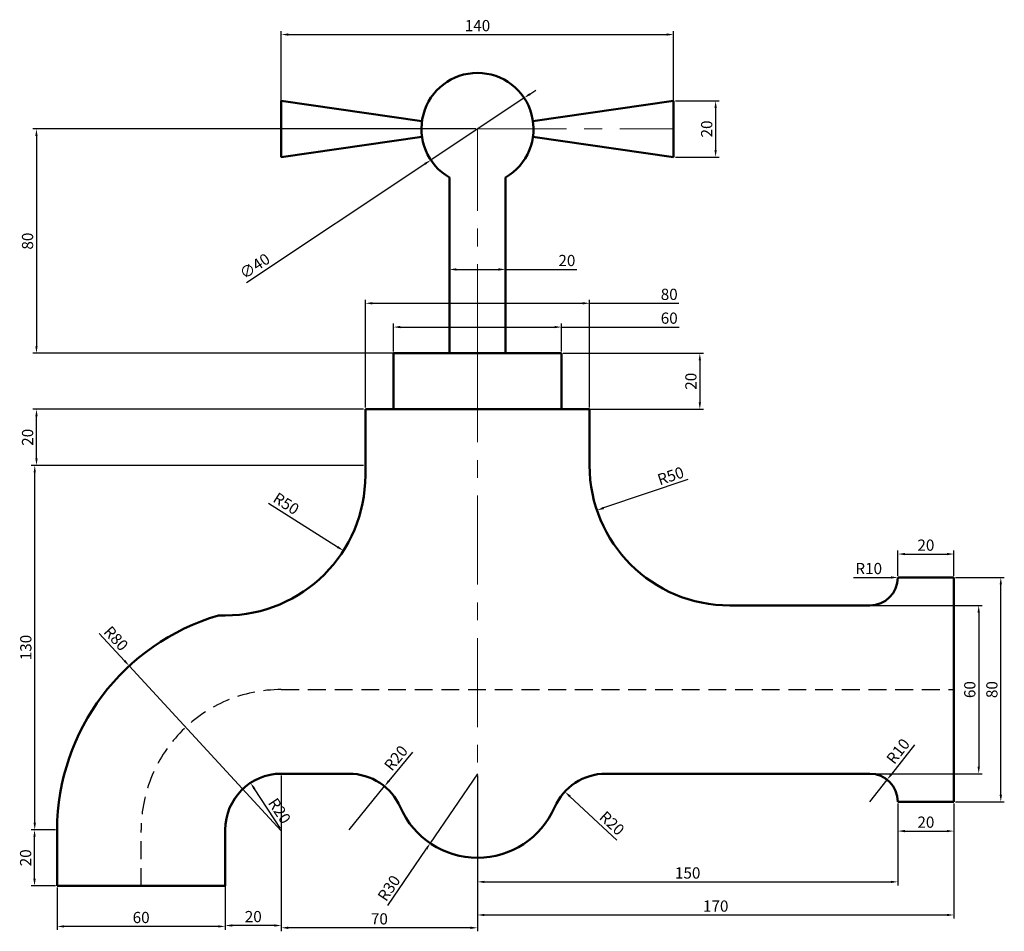
# Model space of a CAD drawing. Units: millimetres. Extents: x 1591 to 1942, y 1200 to 1525.
import ezdxf

# ---------------------------------------------------------------- set-up
doc = ezdxf.new("R2010")
doc.units = ezdxf.units.MM
doc.linetypes.add('CENTER', pattern=[50.8, 31.75, -6.35, 6.35, -6.35])
doc.linetypes.add('HIDDEN', pattern=[9.525, 6.35, -3.175])
for name, color, linetype, lineweight in [('M-CNTR', 1, 'CENTER', 18), ('M-DIMS', 2, 'Continuous', 25), ('M-HIDN', 4, 'HIDDEN', 25), ('M-OUTL', 7, 'Continuous', 50)]:
    doc.layers.add(name, color=color, linetype=linetype, lineweight=lineweight)
doc.styles.get("Standard").update_dxf_attribs({"font": 'arial.ttf'})
doc.dimstyles.new('ISO-25', dxfattribs={"dimtxt": 4, "dimasz": 2.5, "dimexe": 1.25, "dimexo": 0.625, "dimtad": 1, "dimtxsty": 'Standard', "dimcen": 2.5, "dimadec": 0, "dimazin": 0, "dimtfac": 1, "dimtmove": 0, "dimatfit": 3, "dimfxl": 1, "dimarcsym": 0})

# ---------------------------------------------------------------- blocks, each defined once
blk = doc.blocks.new('*D1')
at = {"layer": 'Defpoints', "color": 0, "transparency": 16777216}
for p in [(1923.89, 1325.86), (1940.62, 1325.86), (1923.89, 1245.86)]:
    blk.add_point(p, dxfattribs=at)
at = {"layer": 'M-DIMS', "color": 0, "lineweight": -2, "transparency": 16777216}
for p, q in [((1924.51, 1325.86), (1941.87, 1325.86)), ((1940.62, 1248.36), (1940.62, 1323.36)), ((1924.51, 1245.86), (1941.87, 1245.86))]:
    blk.add_line(p, q, dxfattribs=at)
at = {"layer": 'M-DIMS', "color": 0, "transparency": 16777216}
for points in [[(1940.21, 1323.36), (1941.04, 1323.36), (1940.62, 1325.86)], [(1940.21, 1248.36), (1941.04, 1248.36), (1940.62, 1245.86)]]:
    blk.add_solid(points, dxfattribs=at)
at = {"layer": 'M-DIMS', "color": 0, "transparency": 16777216, "insert": (1937.96, 1285.86), "char_height": 4, "attachment_point": 5, "rotation": 90}
blk.add_mtext('80', dxfattribs=at)
blk = doc.blocks.new('*D2')
at = {"layer": 'Defpoints', "color": 0, "transparency": 16777216}
for p in [(1663.89, 1362.31), (1706.04, 1335.42)]:
    blk.add_point(p, dxfattribs=at)
at = {"layer": 'M-DIMS', "color": 0, "lineweight": -2, "transparency": 16777216}
blk.add_line((1679.37, 1352.43), (1703.94, 1336.76), dxfattribs=at)
at = {"layer": 'M-DIMS', "color": 0, "transparency": 16777216}
blk.add_solid([(1704.16, 1337.11), (1703.71, 1336.41), (1706.04, 1335.42)], dxfattribs=at)
at = {"layer": 'M-DIMS', "color": 0, "transparency": 16777216, "insert": (1685.35, 1351.78), "char_height": 4, "attachment_point": 5, "rotation": 327.4692}
blk.add_mtext('R50', dxfattribs=at)
blk = doc.blocks.new('*D3')
at = {"layer": 'Defpoints', "color": 0, "transparency": 16777216}
for p in [(1843.89, 1365.86), (1796.52, 1349.85)]:
    blk.add_point(p, dxfattribs=at)
at = {"layer": 'M-DIMS', "color": 0, "lineweight": -2, "transparency": 16777216}
blk.add_line((1828.96, 1360.81), (1798.89, 1350.65), dxfattribs=at)
at = {"layer": 'M-DIMS', "color": 0, "transparency": 16777216}
blk.add_solid([(1798.76, 1351.04), (1799.02, 1350.25), (1796.52, 1349.85)], dxfattribs=at)
at = {"layer": 'M-DIMS', "color": 0, "transparency": 16777216, "insert": (1822.99, 1361.61), "char_height": 4, "attachment_point": 5, "rotation": 18.6803}
blk.add_mtext('R50', dxfattribs=at)
blk = doc.blocks.new('*D4')
at = {"layer": 'Defpoints', "color": 0, "transparency": 16777216}
for p in [(1785.05, 1249.46), (1799.71, 1235.86)]:
    blk.add_point(p, dxfattribs=at)
at = {"layer": 'M-DIMS', "color": 0, "lineweight": -2, "transparency": 16777216}
blk.add_line((1803.67, 1232.19), (1786.89, 1247.76), dxfattribs=at)
at = {"layer": 'M-DIMS', "color": 0, "transparency": 16777216}
blk.add_solid([(1787.17, 1248.07), (1786.6, 1247.46), (1785.05, 1249.46)], dxfattribs=at)
at = {"layer": 'M-DIMS', "color": 0, "transparency": 16777216, "insert": (1801.53, 1237.82), "char_height": 4, "attachment_point": 5, "rotation": 317.1429}
blk.add_mtext('R20', dxfattribs=at)
blk = doc.blocks.new('*D5')
at = {"layer": 'Defpoints', "color": 0, "transparency": 16777216}
for p in [(1720.7, 1251.36), (1708.06, 1235.86)]:
    blk.add_point(p, dxfattribs=at)
at = {"layer": 'M-DIMS', "color": 0, "lineweight": -2, "transparency": 16777216}
for p, q in [((1730.68, 1263.6), (1722.28, 1253.3)), ((1708.06, 1235.86), (1720.7, 1251.36))]:
    blk.add_line(p, q, dxfattribs=at)
at = {"layer": 'M-DIMS', "color": 0, "transparency": 16777216}
blk.add_solid([(1721.96, 1253.56), (1722.6, 1253.04), (1720.7, 1251.36)], dxfattribs=at)
at = {"layer": 'M-DIMS', "color": 0, "transparency": 16777216, "insert": (1725.2, 1261.11), "char_height": 4, "attachment_point": 5, "rotation": 50.8113}
blk.add_mtext('R20', dxfattribs=at)
blk = doc.blocks.new('*D6')
at = {"layer": 'Defpoints', "color": 0, "transparency": 16777216}
for p in [(1893.89, 1325.86), (1903.89, 1325.86)]:
    blk.add_point(p, dxfattribs=at)
at = {"layer": 'M-DIMS', "color": 0, "lineweight": -2, "transparency": 16777216}
blk.add_line((1888.09, 1325.86), (1901.39, 1325.86), dxfattribs=at)
at = {"layer": 'M-DIMS', "color": 0, "transparency": 16777216}
blk.add_solid([(1901.39, 1326.28), (1901.39, 1325.44), (1903.89, 1325.86)], dxfattribs=at)
at = {"layer": 'M-DIMS', "color": 0, "transparency": 16777216, "insert": (1893.49, 1328.53), "char_height": 4, "attachment_point": 5}
blk.add_mtext('R10', dxfattribs=at)
blk = doc.blocks.new('*D7')
at = {"layer": 'Defpoints', "color": 0, "transparency": 16777216}
for p in [(1753.89, 1255.86), (1737.03, 1231.05)]:
    blk.add_point(p, dxfattribs=at)
at = {"layer": 'M-DIMS', "color": 0, "lineweight": -2, "transparency": 16777216}
for p, q in [((1753.89, 1255.86), (1737.03, 1231.05)), ((1721.9, 1208.79), (1735.62, 1228.98))]:
    blk.add_line(p, q, dxfattribs=at)
at = {"layer": 'M-DIMS', "color": 0, "transparency": 16777216}
blk.add_solid([(1735.28, 1229.21), (1735.97, 1228.75), (1737.03, 1231.05)], dxfattribs=at)
at = {"layer": 'M-DIMS', "color": 0, "transparency": 16777216, "insert": (1722.73, 1214.75), "char_height": 4, "attachment_point": 5, "rotation": 55.803}
blk.add_mtext('R30', dxfattribs=at)
blk = doc.blocks.new('*D8')
at = {"layer": 'Defpoints', "color": 0, "transparency": 16777216}
for p in [(1672.91, 1252.58), (1683.89, 1235.86)]:
    blk.add_point(p, dxfattribs=at)
at = {"layer": 'M-DIMS', "color": 0, "lineweight": -2, "transparency": 16777216}
blk.add_line((1683.58, 1236.34), (1674.28, 1250.49), dxfattribs=at)
at = {"layer": 'M-DIMS', "color": 0, "transparency": 16777216}
blk.add_solid([(1674.63, 1250.72), (1673.93, 1250.26), (1672.91, 1252.58)], dxfattribs=at)
at = {"layer": 'M-DIMS', "color": 0, "transparency": 16777216, "insert": (1682.84, 1242.31), "char_height": 4, "attachment_point": 5, "rotation": 303.2913}
blk.add_mtext('R20', dxfattribs=at)
blk = doc.blocks.new('*D9')
at = {"layer": 'Defpoints', "color": 0, "transparency": 16777216}
for p in [(1629.63, 1294.31), (1683.89, 1235.52)]:
    blk.add_point(p, dxfattribs=at)
at = {"layer": 'M-DIMS', "color": 0, "lineweight": -2, "transparency": 16777216}
for p, q in [((1618.92, 1305.92), (1627.93, 1296.15)), ((1683.89, 1235.52), (1629.63, 1294.31))]:
    blk.add_line(p, q, dxfattribs=at)
at = {"layer": 'M-DIMS', "color": 0, "transparency": 16777216}
blk.add_solid([(1628.24, 1296.43), (1627.63, 1295.87), (1629.63, 1294.31)], dxfattribs=at)
at = {"layer": 'M-DIMS', "color": 0, "transparency": 16777216, "insert": (1624.54, 1303.76), "char_height": 4, "attachment_point": 5, "rotation": 312.7056}
blk.add_mtext('R80', dxfattribs=at)
blk = doc.blocks.new('*D10')
at = {"layer": 'Defpoints', "color": 0, "transparency": 16777216}
for p in [(1603.89, 1215.86), (1663.89, 1215.86), (1603.89, 1201.38)]:
    blk.add_point(p, dxfattribs=at)
at = {"layer": 'M-DIMS', "color": 0, "lineweight": -2, "transparency": 16777216}
for p, q in [((1603.89, 1215.24), (1603.89, 1200.13)), ((1663.89, 1215.24), (1663.89, 1200.13)), ((1661.39, 1201.38), (1606.39, 1201.38))]:
    blk.add_line(p, q, dxfattribs=at)
at = {"layer": 'M-DIMS', "color": 0, "transparency": 16777216}
for points in [[(1606.39, 1201.8), (1606.39, 1200.97), (1603.89, 1201.38)], [(1661.39, 1201.8), (1661.39, 1200.97), (1663.89, 1201.38)]]:
    blk.add_solid(points, dxfattribs=at)
at = {"layer": 'M-DIMS', "color": 0, "transparency": 16777216, "insert": (1633.89, 1204.05), "char_height": 4, "attachment_point": 5}
blk.add_mtext('60', dxfattribs=at)
blk = doc.blocks.new('*D11')
at = {"layer": 'Defpoints', "color": 0, "transparency": 16777216}
for p in [(1683.89, 1255.86), (1663.89, 1235.86), (1663.89, 1201.7)]:
    blk.add_point(p, dxfattribs=at)
at = {"layer": 'M-DIMS', "color": 0, "lineweight": -2, "transparency": 16777216}
for p, q in [((1683.89, 1255.24), (1683.89, 1200.45)), ((1663.89, 1235.24), (1663.89, 1200.45)), ((1681.39, 1201.7), (1666.39, 1201.7))]:
    blk.add_line(p, q, dxfattribs=at)
at = {"layer": 'M-DIMS', "color": 0, "transparency": 16777216}
for points in [[(1666.39, 1202.12), (1666.39, 1201.29), (1663.89, 1201.7)], [(1681.39, 1202.12), (1681.39, 1201.29), (1683.89, 1201.7)]]:
    blk.add_solid(points, dxfattribs=at)
at = {"layer": 'M-DIMS', "color": 0, "transparency": 16777216, "insert": (1673.89, 1204.37), "char_height": 4, "attachment_point": 5}
blk.add_mtext('20', dxfattribs=at)
blk = doc.blocks.new('*D12')
at = {"layer": 'Defpoints', "color": 0, "transparency": 16777216}
for p in [(1903.89, 1245.86), (1923.89, 1245.86), (1923.89, 1235.39)]:
    blk.add_point(p, dxfattribs=at)
at = {"layer": 'M-DIMS', "color": 0, "lineweight": -2, "transparency": 16777216}
for p, q in [((1903.89, 1245.24), (1903.89, 1234.14)), ((1923.89, 1245.24), (1923.89, 1234.14)), ((1906.39, 1235.39), (1921.39, 1235.39))]:
    blk.add_line(p, q, dxfattribs=at)
at = {"layer": 'M-DIMS', "color": 0, "transparency": 16777216}
for points in [[(1906.39, 1235.81), (1906.39, 1234.98), (1903.89, 1235.39)], [(1921.39, 1235.81), (1921.39, 1234.98), (1923.89, 1235.39)]]:
    blk.add_solid(points, dxfattribs=at)
at = {"layer": 'M-DIMS', "color": 0, "transparency": 16777216, "insert": (1913.89, 1238.06), "char_height": 4, "attachment_point": 5}
blk.add_mtext('20', dxfattribs=at)
blk = doc.blocks.new('*D13')
at = {"layer": 'Defpoints', "color": 0, "transparency": 16777216}
for p in [(1923.89, 1334.22), (1903.89, 1325.86), (1923.89, 1325.86)]:
    blk.add_point(p, dxfattribs=at)
at = {"layer": 'M-DIMS', "color": 0, "lineweight": -2, "transparency": 16777216}
for p, q in [((1903.89, 1326.49), (1903.89, 1335.47)), ((1923.89, 1326.49), (1923.89, 1335.47)), ((1906.39, 1334.22), (1921.39, 1334.22))]:
    blk.add_line(p, q, dxfattribs=at)
at = {"layer": 'M-DIMS', "color": 0, "transparency": 16777216}
for points in [[(1906.39, 1334.63), (1906.39, 1333.8), (1903.89, 1334.22)], [(1921.39, 1334.63), (1921.39, 1333.8), (1923.89, 1334.22)]]:
    blk.add_solid(points, dxfattribs=at)
at = {"layer": 'M-DIMS', "color": 0, "transparency": 16777216, "insert": (1913.89, 1336.88), "char_height": 4, "attachment_point": 5}
blk.add_mtext('20', dxfattribs=at)
blk = doc.blocks.new('*D14')
at = {"layer": 'Defpoints', "color": 0, "transparency": 16777216}
for p in [(1877.49, 1315.86), (1877.49, 1255.86), (1932.74, 1255.86)]:
    blk.add_point(p, dxfattribs=at)
at = {"layer": 'M-DIMS', "color": 0, "lineweight": -2, "transparency": 16777216}
for p, q in [((1878.12, 1315.86), (1933.99, 1315.86)), ((1932.74, 1313.36), (1932.74, 1258.36)), ((1878.12, 1255.86), (1933.99, 1255.86))]:
    blk.add_line(p, q, dxfattribs=at)
at = {"layer": 'M-DIMS', "color": 0, "transparency": 16777216}
for points in [[(1932.32, 1313.36), (1933.15, 1313.36), (1932.74, 1315.86)], [(1932.32, 1258.36), (1933.15, 1258.36), (1932.74, 1255.86)]]:
    blk.add_solid(points, dxfattribs=at)
at = {"layer": 'M-DIMS', "color": 0, "transparency": 16777216, "insert": (1930.07, 1285.86), "char_height": 4, "attachment_point": 5, "rotation": 90}
blk.add_mtext('60', dxfattribs=at)
blk = doc.blocks.new('*D15')
at = {"layer": 'Defpoints', "color": 0, "transparency": 16777216}
for p in [(1900.06, 1253.73), (1893.89, 1245.86)]:
    blk.add_point(p, dxfattribs=at)
at = {"layer": 'M-DIMS', "color": 0, "lineweight": -2, "transparency": 16777216}
for p, q in [((1909.8, 1266.16), (1901.6, 1255.7)), ((1893.89, 1245.86), (1900.06, 1253.73))]:
    blk.add_line(p, q, dxfattribs=at)
at = {"layer": 'M-DIMS', "color": 0, "transparency": 16777216}
blk.add_solid([(1901.27, 1255.96), (1901.93, 1255.44), (1900.06, 1253.73)], dxfattribs=at)
at = {"layer": 'M-DIMS', "color": 0, "transparency": 16777216, "insert": (1904.37, 1263.56), "char_height": 4, "attachment_point": 5, "rotation": 51.9172}
blk.add_mtext('R10', dxfattribs=at)
blk = doc.blocks.new('*D16')
at = {"layer": 'Defpoints', "color": 0, "transparency": 16777216}
for p in [(1753.89, 1255.86), (1923.89, 1245.86), (1923.89, 1205.46)]:
    blk.add_point(p, dxfattribs=at)
at = {"layer": 'M-DIMS', "color": 0, "lineweight": -2, "transparency": 16777216}
for p, q in [((1753.89, 1255.24), (1753.89, 1204.21)), ((1923.89, 1245.24), (1923.89, 1204.21)), ((1756.39, 1205.46), (1921.39, 1205.46))]:
    blk.add_line(p, q, dxfattribs=at)
at = {"layer": 'M-DIMS', "color": 0, "transparency": 16777216}
for points in [[(1756.39, 1205.87), (1756.39, 1205.04), (1753.89, 1205.46)], [(1921.39, 1205.87), (1921.39, 1205.04), (1923.89, 1205.46)]]:
    blk.add_solid(points, dxfattribs=at)
at = {"layer": 'M-DIMS', "color": 0, "transparency": 16777216, "insert": (1838.89, 1208.12), "char_height": 4, "attachment_point": 5}
blk.add_mtext('170', dxfattribs=at)
blk = doc.blocks.new('*D17')
at = {"layer": 'Defpoints', "color": 0, "transparency": 16777216}
for p in [(1753.89, 1255.86), (1903.89, 1245.86), (1903.89, 1217.27)]:
    blk.add_point(p, dxfattribs=at)
at = {"layer": 'M-DIMS', "color": 0, "lineweight": -2, "transparency": 16777216}
for p, q in [((1753.89, 1255.24), (1753.89, 1216.02)), ((1903.89, 1245.24), (1903.89, 1216.02)), ((1756.39, 1217.27), (1901.39, 1217.27))]:
    blk.add_line(p, q, dxfattribs=at)
at = {"layer": 'M-DIMS', "color": 0, "transparency": 16777216}
for points in [[(1756.39, 1217.68), (1756.39, 1216.85), (1753.89, 1217.27)], [(1901.39, 1217.68), (1901.39, 1216.85), (1903.89, 1217.27)]]:
    blk.add_solid(points, dxfattribs=at)
at = {"layer": 'M-DIMS', "color": 0, "transparency": 16777216, "insert": (1828.89, 1219.93), "char_height": 4, "attachment_point": 5}
blk.add_mtext('150', dxfattribs=at)
blk = doc.blocks.new('*D18')
at = {"layer": 'Defpoints', "color": 0, "transparency": 16777216}
for p in [(1683.89, 1255.86), (1753.89, 1255.86), (1683.89, 1200.89)]:
    blk.add_point(p, dxfattribs=at)
at = {"layer": 'M-DIMS', "color": 0, "lineweight": -2, "transparency": 16777216}
for p, q in [((1683.89, 1255.24), (1683.89, 1199.64)), ((1753.89, 1255.24), (1753.89, 1199.64)), ((1751.39, 1200.89), (1686.39, 1200.89))]:
    blk.add_line(p, q, dxfattribs=at)
at = {"layer": 'M-DIMS', "color": 0, "transparency": 16777216}
for points in [[(1686.39, 1201.3), (1686.39, 1200.47), (1683.89, 1200.89)], [(1751.39, 1201.3), (1751.39, 1200.47), (1753.89, 1200.89)]]:
    blk.add_solid(points, dxfattribs=at)
at = {"layer": 'M-DIMS', "color": 0, "transparency": 16777216, "insert": (1718.89, 1203.56), "char_height": 4, "attachment_point": 5}
blk.add_mtext('70', dxfattribs=at)
blk = doc.blocks.new('*D19')
at = {"layer": 'Defpoints', "color": 0, "transparency": 16777216}
for p in [(1595.83, 1235.86), (1603.89, 1235.86), (1603.89, 1215.86)]:
    blk.add_point(p, dxfattribs=at)
at = {"layer": 'M-DIMS', "color": 0, "lineweight": -2, "transparency": 16777216}
for p, q in [((1603.26, 1235.86), (1594.58, 1235.86)), ((1595.83, 1218.36), (1595.83, 1233.36)), ((1603.26, 1215.86), (1594.58, 1215.86))]:
    blk.add_line(p, q, dxfattribs=at)
at = {"layer": 'M-DIMS', "color": 0, "transparency": 16777216}
for points in [[(1595.42, 1233.36), (1596.25, 1233.36), (1595.83, 1235.86)], [(1595.42, 1218.36), (1596.25, 1218.36), (1595.83, 1215.86)]]:
    blk.add_solid(points, dxfattribs=at)
at = {"layer": 'M-DIMS', "color": 0, "transparency": 16777216, "insert": (1593.17, 1225.86), "char_height": 4, "attachment_point": 5, "rotation": 90}
blk.add_mtext('20', dxfattribs=at)
blk = doc.blocks.new('*D20')
at = {"layer": 'Defpoints', "color": 0, "transparency": 16777216}
for p in [(1595.92, 1365.86), (1713.89, 1365.86), (1603.89, 1235.86)]:
    blk.add_point(p, dxfattribs=at)
at = {"layer": 'M-DIMS', "color": 0, "lineweight": -2, "transparency": 16777216}
for p, q in [((1713.26, 1365.86), (1594.67, 1365.86)), ((1595.92, 1238.36), (1595.92, 1363.36)), ((1603.26, 1235.86), (1594.67, 1235.86))]:
    blk.add_line(p, q, dxfattribs=at)
at = {"layer": 'M-DIMS', "color": 0, "transparency": 16777216}
for points in [[(1595.5, 1363.36), (1596.33, 1363.36), (1595.92, 1365.86)], [(1595.5, 1238.36), (1596.33, 1238.36), (1595.92, 1235.86)]]:
    blk.add_solid(points, dxfattribs=at)
at = {"layer": 'M-DIMS', "color": 0, "transparency": 16777216, "insert": (1593.25, 1300.86), "char_height": 4, "attachment_point": 5, "rotation": 90}
blk.add_mtext('130', dxfattribs=at)
blk = doc.blocks.new('*D21')
at = {"layer": 'Defpoints', "color": 0, "transparency": 16777216}
for p in [(1596.54, 1385.86), (1713.89, 1385.86), (1713.89, 1365.86)]:
    blk.add_point(p, dxfattribs=at)
at = {"layer": 'M-DIMS', "color": 0, "lineweight": -2, "transparency": 16777216}
for p, q in [((1713.26, 1385.86), (1595.29, 1385.86)), ((1596.54, 1368.36), (1596.54, 1383.36)), ((1713.26, 1365.86), (1595.29, 1365.86))]:
    blk.add_line(p, q, dxfattribs=at)
at = {"layer": 'M-DIMS', "color": 0, "transparency": 16777216}
for points in [[(1596.13, 1383.36), (1596.96, 1383.36), (1596.54, 1385.86)], [(1596.13, 1368.36), (1596.96, 1368.36), (1596.54, 1365.86)]]:
    blk.add_solid(points, dxfattribs=at)
at = {"layer": 'M-DIMS', "color": 0, "transparency": 16777216, "insert": (1593.87, 1375.86), "char_height": 4, "attachment_point": 5, "rotation": 90}
blk.add_mtext('20', dxfattribs=at)
blk = doc.blocks.new('*D22')
at = {"layer": 'Defpoints', "color": 0, "transparency": 16777216}
for p in [(1783.89, 1405.86), (1783.89, 1385.86), (1833.23, 1385.86)]:
    blk.add_point(p, dxfattribs=at)
at = {"layer": 'M-DIMS', "color": 0, "lineweight": -2, "transparency": 16777216}
for p, q in [((1784.51, 1405.86), (1834.48, 1405.86)), ((1833.23, 1403.36), (1833.23, 1388.36)), ((1784.51, 1385.86), (1834.48, 1385.86))]:
    blk.add_line(p, q, dxfattribs=at)
at = {"layer": 'M-DIMS', "color": 0, "transparency": 16777216}
for points in [[(1832.81, 1403.36), (1833.65, 1403.36), (1833.23, 1405.86)], [(1832.81, 1388.36), (1833.65, 1388.36), (1833.23, 1385.86)]]:
    blk.add_solid(points, dxfattribs=at)
at = {"layer": 'M-DIMS', "color": 0, "transparency": 16777216, "insert": (1830.56, 1395.86), "char_height": 4, "attachment_point": 5, "rotation": 90}
blk.add_mtext('20', dxfattribs=at)
blk = doc.blocks.new('*D23')
at = {"layer": 'Defpoints', "color": 0, "transparency": 16777216}
for p in [(1793.89, 1423.68), (1713.89, 1385.86), (1793.89, 1385.86)]:
    blk.add_point(p, dxfattribs=at)
at = {"layer": 'M-DIMS', "color": 0, "lineweight": -2, "transparency": 16777216}
for p, q in [((1713.89, 1386.49), (1713.89, 1424.93)), ((1716.39, 1423.68), (1791.39, 1423.68)), ((1793.89, 1386.49), (1793.89, 1424.93)), ((1793.89, 1423.68), (1825.79, 1423.68))]:
    blk.add_line(p, q, dxfattribs=at)
at = {"layer": 'M-DIMS', "color": 0, "transparency": 16777216}
for points in [[(1716.39, 1424.1), (1716.39, 1423.26), (1713.89, 1423.68)], [(1791.39, 1424.1), (1791.39, 1423.26), (1793.89, 1423.68)]]:
    blk.add_solid(points, dxfattribs=at)
at = {"layer": 'M-DIMS', "color": 0, "transparency": 16777216, "insert": (1822.31, 1426.35), "char_height": 4, "attachment_point": 5}
blk.add_mtext('80', dxfattribs=at)
blk = doc.blocks.new('*D24')
at = {"layer": 'Defpoints', "color": 0, "transparency": 16777216}
for p in [(1783.89, 1415.19), (1723.89, 1405.86), (1783.89, 1405.86)]:
    blk.add_point(p, dxfattribs=at)
at = {"layer": 'M-DIMS', "color": 0, "lineweight": -2, "transparency": 16777216}
for p, q in [((1723.89, 1406.49), (1723.89, 1416.44)), ((1783.89, 1406.49), (1783.89, 1416.44)), ((1726.39, 1415.19), (1781.39, 1415.19)), ((1783.89, 1415.19), (1825.8, 1415.19))]:
    blk.add_line(p, q, dxfattribs=at)
at = {"layer": 'M-DIMS', "color": 0, "transparency": 16777216}
for points in [[(1726.39, 1415.61), (1726.39, 1414.78), (1723.89, 1415.19)], [(1781.39, 1415.61), (1781.39, 1414.78), (1783.89, 1415.19)]]:
    blk.add_solid(points, dxfattribs=at)
at = {"layer": 'M-DIMS', "color": 0, "transparency": 16777216, "insert": (1822.31, 1417.86), "char_height": 4, "attachment_point": 5}
blk.add_mtext('60', dxfattribs=at)
blk = doc.blocks.new('*D25')
at = {"layer": 'Defpoints', "color": 0, "transparency": 16777216}
for p in [(1743.89, 1448.72), (1763.89, 1448.72), (1763.89, 1435.75)]:
    blk.add_point(p, dxfattribs=at)
at = {"layer": 'M-DIMS', "color": 0, "lineweight": -2, "transparency": 16777216}
for p, q in [((1743.89, 1448.09), (1743.89, 1434.5)), ((1763.89, 1448.09), (1763.89, 1434.5)), ((1746.39, 1435.75), (1761.39, 1435.75)), ((1763.89, 1435.75), (1789.31, 1435.75))]:
    blk.add_line(p, q, dxfattribs=at)
at = {"layer": 'M-DIMS', "color": 0, "transparency": 16777216}
for points in [[(1746.39, 1436.17), (1746.39, 1435.33), (1743.89, 1435.75)], [(1761.39, 1436.17), (1761.39, 1435.33), (1763.89, 1435.75)]]:
    blk.add_solid(points, dxfattribs=at)
at = {"layer": 'M-DIMS', "color": 0, "transparency": 16777216, "insert": (1785.79, 1438.42), "char_height": 4, "attachment_point": 5}
blk.add_mtext('20', dxfattribs=at)
blk = doc.blocks.new('*D26')
at = {"layer": 'Defpoints', "color": 0, "transparency": 16777216}
for p in [(1770.54, 1496.94), (1737.24, 1474.78)]:
    blk.add_point(p, dxfattribs=at)
at = {"layer": 'M-DIMS', "color": 0, "lineweight": -2, "transparency": 16777216}
for p, q in [((1770.54, 1496.94), (1737.24, 1474.78)), ((1772.62, 1498.32), (1774.7, 1499.71)), ((1671.52, 1431.06), (1735.16, 1473.4))]:
    blk.add_line(p, q, dxfattribs=at)
at = {"layer": 'M-DIMS', "color": 0, "transparency": 16777216}
for points in [[(1772.39, 1498.67), (1772.85, 1497.98), (1770.54, 1496.94)], [(1734.92, 1473.75), (1735.39, 1473.05), (1737.24, 1474.78)]]:
    blk.add_solid(points, dxfattribs=at)
at = {"layer": 'M-DIMS', "color": 0, "transparency": 16777216, "insert": (1674.69, 1436.51), "char_height": 4, "attachment_point": 5, "rotation": 33.6324}
blk.add_mtext('∅40', dxfattribs=at)
blk = doc.blocks.new('*D27')
at = {"layer": 'Defpoints', "color": 0, "transparency": 16777216}
for p in [(1753.89, 1485.86), (1596.52, 1405.86), (1753.89, 1405.86)]:
    blk.add_point(p, dxfattribs=at)
at = {"layer": 'M-DIMS', "color": 0, "lineweight": -2, "transparency": 16777216}
for p, q in [((1753.26, 1485.86), (1595.27, 1485.86)), ((1596.52, 1483.36), (1596.52, 1408.36)), ((1753.26, 1405.86), (1595.27, 1405.86))]:
    blk.add_line(p, q, dxfattribs=at)
at = {"layer": 'M-DIMS', "color": 0, "transparency": 16777216}
for points in [[(1596.11, 1483.36), (1596.94, 1483.36), (1596.52, 1485.86)], [(1596.11, 1408.36), (1596.94, 1408.36), (1596.52, 1405.86)]]:
    blk.add_solid(points, dxfattribs=at)
at = {"layer": 'M-DIMS', "color": 0, "transparency": 16777216, "insert": (1593.86, 1445.86), "char_height": 4, "attachment_point": 5, "rotation": 90}
blk.add_mtext('80', dxfattribs=at)
blk = doc.blocks.new('*D28')
at = {"layer": 'Defpoints', "color": 0, "transparency": 16777216}
for p in [(1823.89, 1519.55), (1683.89, 1485.86), (1823.89, 1485.86)]:
    blk.add_point(p, dxfattribs=at)
at = {"layer": 'M-DIMS', "color": 0, "lineweight": -2, "transparency": 16777216}
for p, q in [((1683.89, 1486.49), (1683.89, 1520.8)), ((1686.39, 1519.55), (1821.39, 1519.55)), ((1823.89, 1486.49), (1823.89, 1520.8))]:
    blk.add_line(p, q, dxfattribs=at)
at = {"layer": 'M-DIMS', "color": 0, "transparency": 16777216}
for points in [[(1686.39, 1519.97), (1686.39, 1519.14), (1683.89, 1519.55)], [(1821.39, 1519.97), (1821.39, 1519.14), (1823.89, 1519.55)]]:
    blk.add_solid(points, dxfattribs=at)
at = {"layer": 'M-DIMS', "color": 0, "transparency": 16777216, "insert": (1753.89, 1522.22), "char_height": 4, "attachment_point": 5}
blk.add_mtext('140', dxfattribs=at)
blk = doc.blocks.new('*D29')
at = {"layer": 'Defpoints', "color": 0, "transparency": 16777216}
for p in [(1823.89, 1495.86), (1823.89, 1475.86), (1838.86, 1475.86)]:
    blk.add_point(p, dxfattribs=at)
at = {"layer": 'M-DIMS', "color": 0, "lineweight": -2, "transparency": 16777216}
for p, q in [((1824.51, 1495.86), (1840.11, 1495.86)), ((1838.86, 1493.36), (1838.86, 1478.36)), ((1824.51, 1475.86), (1840.11, 1475.86))]:
    blk.add_line(p, q, dxfattribs=at)
at = {"layer": 'M-DIMS', "color": 0, "transparency": 16777216}
for points in [[(1838.44, 1493.36), (1839.27, 1493.36), (1838.86, 1495.86)], [(1838.44, 1478.36), (1839.27, 1478.36), (1838.86, 1475.86)]]:
    blk.add_solid(points, dxfattribs=at)
at = {"layer": 'M-DIMS', "color": 0, "transparency": 16777216, "insert": (1836.19, 1485.86), "char_height": 4, "attachment_point": 5, "rotation": 90}
blk.add_mtext('20', dxfattribs=at)

msp = doc.modelspace()

# ---------------------------------------------------------------- linework, layer by layer
at = {"layer": 'M-CNTR'}
for p, q in [((1753.889, 1405.861), (1753.889, 1485.861)), ((1753.889, 1485.861), (1823.889, 1485.861)), ((1753.889, 1405.861), (1753.889, 1225.861))]:
    msp.add_line(p, q, dxfattribs=at)
at = {"layer": 'M-HIDN'}
for p, q in [((1683.889, 1285.861), (1923.889, 1285.861)), ((1633.889, 1215.861), (1633.889, 1235.861))]:
    msp.add_line(p, q, dxfattribs=at)
msp.add_arc((1683.889, 1235.861), 50, 90, 180, dxfattribs=at)
at = {"layer": 'M-OUTL'}
for p, q in [((1683.889, 1485.861), (1683.889, 1495.861)), ((1683.889, 1495.861), (1734.09, 1488.689)), ((1823.889, 1495.861), (1773.688, 1488.689)), ((1823.889, 1485.861), (1823.889, 1495.861)), ((1683.889, 1485.861), (1683.889, 1475.861)), ((1683.889, 1475.861), (1734.09, 1483.032)), ((1823.889, 1475.861), (1773.688, 1483.032)), ((1823.889, 1485.861), (1823.889, 1475.861)), ((1743.889, 1468.54), (1743.889, 1405.861)), ((1763.889, 1405.861), (1763.889, 1468.54)), ((1783.889, 1405.861), (1723.889, 1405.861)), ((1723.889, 1405.861), (1723.889, 1385.861)), ((1783.889, 1385.861), (1783.889, 1405.861)), ((1753.889, 1385.861), (1713.889, 1385.861)), ((1713.889, 1385.861), (1713.889, 1365.861)), ((1753.889, 1385.861), (1793.889, 1385.861)), ((1793.889, 1385.861), (1793.889, 1365.861)), ((1713.889, 1362.307), (1713.889, 1365.861)), ((1793.889, 1365.861), (1793.889, 1365.861)), ((1923.889, 1325.861), (1903.889, 1325.861)), ((1903.889, 1325.861), (1903.889, 1325.861)), ((1923.889, 1245.861), (1923.889, 1325.861)), ((1843.889, 1315.861), (1893.889, 1315.861)), ((1661.432, 1312.307), (1663.889, 1312.307)), ((1708.063, 1255.861), (1683.889, 1255.861)), ((1799.715, 1255.861), (1893.889, 1255.861)), ((1903.889, 1245.861), (1903.889, 1245.861)), ((1903.889, 1245.861), (1923.889, 1245.861)), ((1603.889, 1215.861), (1603.889, 1235.861)), ((1663.889, 1235.861), (1663.889, 1235.861)), ((1663.889, 1235.861), (1663.889, 1215.861)), ((1663.889, 1215.861), (1603.889, 1215.861))]:
    msp.add_line(p, q, dxfattribs=at)
for centre, radius, start, end in [((1753.889, 1485.861), 20, 300, 240), ((1843.889, 1365.861), 50, 180, 270), ((1663.889, 1362.307), 50, 270, 0), ((1893.889, 1325.861), 10, 270, 0), ((1683.888, 1235.523), 80, 106.30171, 179.75787), ((1683.889, 1235.861), 20, 90, 180), ((1708.063, 1235.861), 20, 23.57818, 90), ((1799.715, 1235.861), 20, 90, 156.42182), ((1893.889, 1245.861), 10, 0, 90), ((1753.889, 1255.861), 30, 203.57818, 336.42182)]:
    msp.add_arc(centre, radius, start, end, dxfattribs=at)

# ---------------------------------------------------------------- dimensions: what is measured, and where the dimension line sits
at = {"layer": 'M-DIMS'}
for base, p1, p2, picture, middle in [((1823.889, 1519.553), (1683.889, 1485.861), (1823.889, 1485.861), '*D28', (1753.889, 1522.22)), ((1923.889, 1334.218), (1903.889, 1325.861), (1923.889, 1325.861), '*D13', (1913.889, 1336.885)), ((1663.889, 1201.703), (1683.889, 1255.861), (1663.889, 1235.861), '*D11', (1673.889, 1204.37)), ((1683.889, 1200.888), (1753.889, 1255.861), (1683.889, 1255.861), '*D18', (1718.889, 1203.555)), ((1923.889, 1205.456), (1753.889, 1255.861), (1923.889, 1245.861), '*D16', (1838.889, 1208.123)), ((1903.889, 1217.266), (1753.889, 1255.861), (1903.889, 1245.861), '*D17', (1828.889, 1219.934)), ((1923.889, 1235.393), (1903.889, 1245.861), (1923.889, 1245.861), '*D12', (1913.889, 1238.06)), ((1603.889, 1201.382), (1663.889, 1215.861), (1603.889, 1215.861), '*D10', (1633.889, 1204.049))]:
    dim = msp.add_linear_dim(base=base, p1=p1, p2=p2, dimstyle='ISO-25', override={"dimclrd": 0, "dimclre": 0, "dimclrt": 0}, dxfattribs=at)
    dim.commit()
    dim.dimension.update_dxf_attribs({"geometry": picture, "text_midpoint": middle})
dim = msp.add_diameter_dim_2p(p1=(1770.541, 1496.938), p2=(1737.237, 1474.784), dimstyle='ISO-25', override={"dimclrd": 0, "dimclre": 0, "dimclrt": 0}, dxfattribs=at)
dim.commit()
dim.dimension.update_dxf_attribs({"geometry": '*D26', "text_midpoint": (1676.227, 1434.199), "dimtype": 163})
for base, p1, p2, picture, middle in [((1838.856, 1475.861), (1823.889, 1495.861), (1823.889, 1475.861), '*D29', (1836.189, 1485.861)), ((1596.523, 1405.861), (1753.889, 1485.861), (1753.889, 1405.861), '*D27', (1593.855, 1445.861)), ((1833.23, 1385.861), (1783.889, 1405.861), (1783.889, 1385.861), '*D22', (1830.563, 1395.861)), ((1596.542, 1385.861), (1713.889, 1365.861), (1713.889, 1385.861), '*D21', (1593.875, 1375.861)), ((1595.916, 1365.861), (1603.889, 1235.861), (1713.889, 1365.861), '*D20', (1593.248, 1300.861)), ((1940.623, 1325.861), (1923.889, 1245.861), (1923.889, 1325.861), '*D1', (1937.956, 1285.861)), ((1932.735, 1255.861), (1877.493, 1315.861), (1877.493, 1255.861), '*D14', (1930.068, 1285.861)), ((1595.834, 1235.861), (1603.889, 1215.861), (1603.889, 1235.861), '*D19', (1593.167, 1225.861))]:
    dim = msp.add_linear_dim(base=base, p1=p1, p2=p2, angle=90, dimstyle='ISO-25', override={"dimclrd": 0, "dimclre": 0, "dimclrt": 0}, dxfattribs=at)
    dim.commit()
    dim.dimension.update_dxf_attribs({"geometry": picture, "text_midpoint": middle})
for base, p1, p2, picture, middle in [((1763.889, 1435.75), (1743.889, 1448.719), (1763.889, 1448.719), '*D25', (1785.788, 1435.75)), ((1793.889, 1423.678), (1713.889, 1385.861), (1793.889, 1385.861), '*D23', (1822.308, 1423.678)), ((1783.889, 1415.194), (1723.889, 1405.861), (1783.889, 1405.861), '*D24', (1822.308, 1415.194))]:
    dim = msp.add_linear_dim(base=base, p1=p1, p2=p2, dimstyle='ISO-25', override={"dimclrd": 0, "dimclre": 0, "dimclrt": 0}, dxfattribs=at)
    dim.commit()
    dim.dimension.update_dxf_attribs({"geometry": picture, "text_midpoint": middle, "dimtype": 160})
for center, mpoint, picture, middle in [((1843.889, 1365.861), (1796.523, 1349.847), '*D3', (1823.848, 1359.085)), ((1663.889, 1362.307), (1706.044, 1335.419), '*D2', (1683.919, 1349.531)), ((1893.889, 1325.861), (1903.889, 1325.861), '*D6', (1893.492, 1325.861)), ((1753.889, 1255.861), (1737.028, 1231.048), '*D7', (1724.936, 1213.254)), ((1683.889, 1235.861), (1672.911, 1252.579), '*D8', (1680.614, 1240.847)), ((1799.715, 1235.861), (1785.054, 1249.464), '*D4', (1799.715, 1235.861))]:
    dim = msp.add_radius_dim(center=center, mpoint=mpoint, dimstyle='ISO-25', override={"dimclrd": 0, "dimclre": 0, "dimclrt": 0}, dxfattribs=at)
    dim.commit()
    dim.dimension.update_dxf_attribs({"geometry": picture, "text_midpoint": middle, "dimtype": 164})
for center, mpoint, picture, middle in [((1683.888, 1235.523), (1629.63, 1294.311), '*D9', (1624.538, 1303.76)), ((1893.889, 1245.861), (1900.057, 1253.732), '*D15', (1904.37, 1263.561)), ((1708.063, 1235.861), (1720.701, 1251.362), '*D5', (1725.203, 1261.106))]:
    dim = msp.add_radius_dim(center=center, mpoint=mpoint, dimstyle='ISO-25', override={"dimclrd": 0, "dimclre": 0, "dimclrt": 0}, dxfattribs=at)
    dim.commit()
    dim.dimension.update_dxf_attribs({"geometry": picture, "text_midpoint": middle})

doc.saveas('drawing.dxf')
